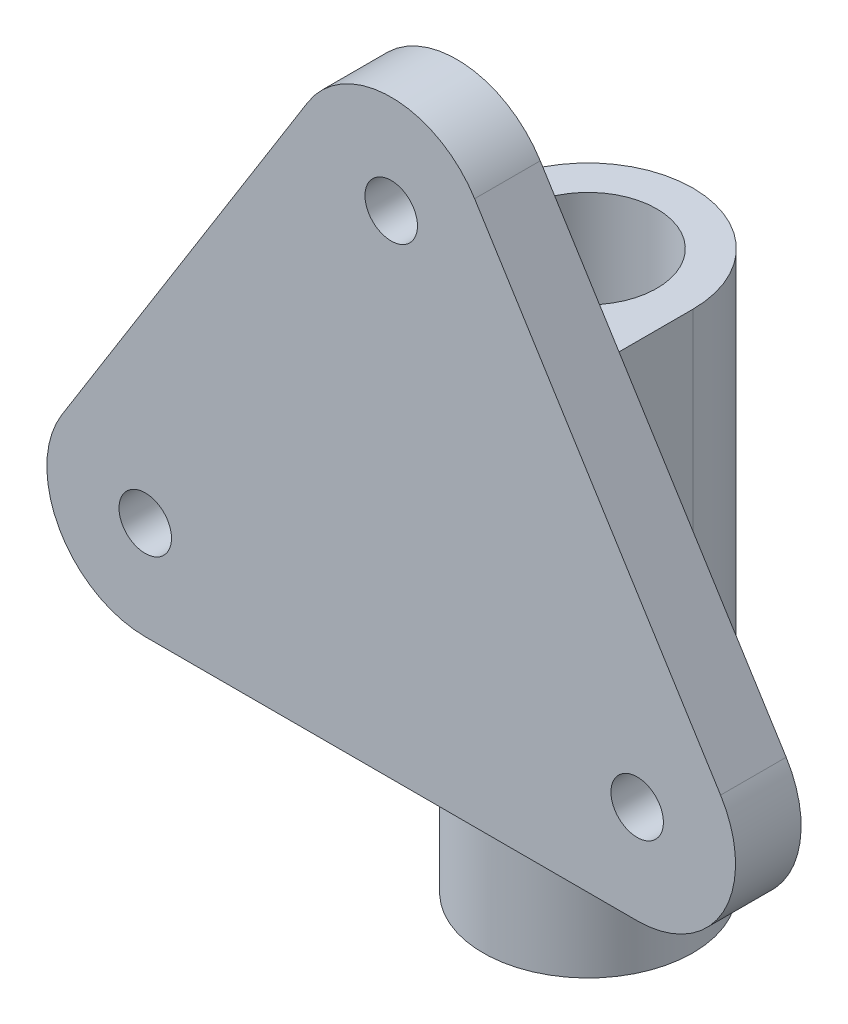
ISO-10303-21;
HEADER;
FILE_DESCRIPTION(('STEP AP214'),'2;1');
FILE_NAME('part.step','',(''),(''),'','','');
FILE_SCHEMA(('AUTOMOTIVE_DESIGN { 1 0 10303 214 1 1 1 1 }'));
ENDSEC;
DATA;
#1=APPLICATION_CONTEXT('core data for automotive mechanical design processes');
#2=APPLICATION_PROTOCOL_DEFINITION('international standard','automotive_design',2000,#1);
#3=PRODUCT_CONTEXT('',#1,'mechanical');
#4=PRODUCT('Part','Part','',(#3));
#5=PRODUCT_RELATED_PRODUCT_CATEGORY('part','',(#4));
#6=PRODUCT_DEFINITION_FORMATION('','',#4);
#7=PRODUCT_DEFINITION_CONTEXT('part definition',#1,'design');
#8=PRODUCT_DEFINITION('design','',#6,#7);
#9=PRODUCT_DEFINITION_SHAPE('','',#8);
#10=(LENGTH_UNIT() NAMED_UNIT(*) SI_UNIT(.MILLI.,.METRE.));
#11=(NAMED_UNIT(*) PLANE_ANGLE_UNIT() SI_UNIT($,.RADIAN.));
#12=(NAMED_UNIT(*) SI_UNIT($,.STERADIAN.) SOLID_ANGLE_UNIT());
#13=UNCERTAINTY_MEASURE_WITH_UNIT(LENGTH_MEASURE(1.E-05),#10,'distance_accuracy_value','');
#14=(GEOMETRIC_REPRESENTATION_CONTEXT(3) GLOBAL_UNCERTAINTY_ASSIGNED_CONTEXT((#13)) GLOBAL_UNIT_ASSIGNED_CONTEXT((#10,
#11,#12)) REPRESENTATION_CONTEXT('',''));
#15=CARTESIAN_POINT('',(0.,0.,0.));
#16=DIRECTION('',(0.,0.,1.));
#17=DIRECTION('',(1.,0.,0.));
#18=AXIS2_PLACEMENT_3D('',#15,#16,#17);
#19=CARTESIAN_POINT('',(-16.,-105.,0.));
#20=DIRECTION('',(1.,0.,0.));
#21=DIRECTION('',(0.,0.,-1.));
#22=AXIS2_PLACEMENT_3D('',#19,#20,#21);
#23=PLANE('',#22);
#24=DIRECTION('',(0.,0.,-1.));
#25=VECTOR('',#24,1.);
#26=CARTESIAN_POINT('',(-16.,-75.,0.));
#27=LINE('',#26,#25);
#28=CARTESIAN_POINT('',(-16.,-75.,0.));
#29=VERTEX_POINT('',#28);
#30=CARTESIAN_POINT('',(-16.,-75.,-20.));
#31=VERTEX_POINT('',#30);
#32=EDGE_CURVE('E191',#29,#31,#27,.T.);
#33=ORIENTED_EDGE('',*,*,#32,.F.);
#34=DIRECTION('',(0.,1.,0.));
#35=VECTOR('',#34,1.);
#36=CARTESIAN_POINT('',(-16.,-60.,0.));
#37=LINE('',#36,#35);
#38=CARTESIAN_POINT('',(-16.,-20.,0.));
#39=VERTEX_POINT('',#38);
#40=EDGE_CURVE('E207',#29,#39,#37,.T.);
#41=ORIENTED_EDGE('',*,*,#40,.T.);
#42=DIRECTION('',(0.,0.,-1.));
#43=VECTOR('',#42,1.);
#44=CARTESIAN_POINT('',(-16.,-20.,0.));
#45=LINE('',#44,#43);
#46=CARTESIAN_POINT('',(-16.,-20.,-20.));
#47=VERTEX_POINT('',#46);
#48=EDGE_CURVE('E232',#39,#47,#45,.T.);
#49=ORIENTED_EDGE('',*,*,#48,.T.);
#50=DIRECTION('',(0.,1.,0.));
#51=VECTOR('',#50,1.);
#52=CARTESIAN_POINT('',(-16.,-105.,-20.));
#53=LINE('',#52,#51);
#54=EDGE_CURVE('E209',#31,#47,#53,.T.);
#55=ORIENTED_EDGE('',*,*,#54,.F.);
#56=EDGE_LOOP('',(#33,#41,#49,#55));
#57=FACE_BOUND('',#56,.T.);
#58=ADVANCED_FACE('F102',(#57),#23,.F.);
#59=CARTESIAN_POINT('',(0.,-105.,0.));
#60=DIRECTION('',(0.,-1.,0.));
#61=DIRECTION('',(0.,0.,-1.));
#62=AXIS2_PLACEMENT_3D('',#59,#60,#61);
#63=PLANE('',#62);
#64=CARTESIAN_POINT('',(0.,-105.,-20.));
#65=DIRECTION('',(0.,-1.,0.));
#66=DIRECTION('',(0.,0.,-1.));
#67=AXIS2_PLACEMENT_3D('',#64,#65,#66);
#68=CIRCLE('',#67,10.5);
#69=CARTESIAN_POINT('',(0.,-105.,-30.5));
#70=VERTEX_POINT('',#69);
#71=EDGE_CURVE('E231',#70,#70,#68,.T.);
#72=ORIENTED_EDGE('',*,*,#71,.F.);
#73=EDGE_LOOP('',(#72));
#74=FACE_BOUND('',#73,.T.);
#75=CARTESIAN_POINT('',(0.,-105.,-20.));
#76=DIRECTION('',(0.,-1.,0.));
#77=DIRECTION('',(0.,0.,-1.));
#78=AXIS2_PLACEMENT_3D('',#75,#76,#77);
#79=CIRCLE('',#78,16.);
#80=CARTESIAN_POINT('',(-16.,-105.,-20.));
#81=VERTEX_POINT('',#80);
#82=CARTESIAN_POINT('',(16.,-105.,-20.));
#83=VERTEX_POINT('',#82);
#84=EDGE_CURVE('E213',#81,#83,#79,.T.);
#85=ORIENTED_EDGE('',*,*,#84,.T.);
#86=CARTESIAN_POINT('',(16.,-105.,-20.));
#87=CARTESIAN_POINT('',(16.,-105.,-16.8176750296418));
#88=CARTESIAN_POINT('',(14.7820725201806,-105.,-13.8770650821586));
#89=CARTESIAN_POINT('',(13.5644424143641,-105.,-10.9371731256605));
#90=CARTESIAN_POINT('',(11.3137084989848,-105.,-8.68629150101524));
#91=CARTESIAN_POINT('',(9.06371702136959,-105.,-6.43615236285823));
#92=CARTESIAN_POINT('',(6.12293491784144,-105.,-5.21792747981942));
#93=CARTESIAN_POINT('',(3.18312287464358,-105.,-4.00010444621753));
#94=CARTESIAN_POINT('',(0.,-105.,-4.));
#95=CARTESIAN_POINT('',(-3.18207287466311,-105.,-3.9998955882356));
#96=CARTESIAN_POINT('',(-6.12293491784143,-105.,-5.21792747981941));
#97=CARTESIAN_POINT('',(-9.0628268743386,-105.,-6.435557585635));
#98=CARTESIAN_POINT('',(-11.3137084989848,-105.,-8.68629150101524));
#99=CARTESIAN_POINT('',(-13.5638476371406,-105.,-10.9362829786292));
#100=CARTESIAN_POINT('',(-14.7820725201806,-105.,-13.8770650821586));
#101=CARTESIAN_POINT('',(-16.,-105.,-16.8171292574295));
#102=CARTESIAN_POINT('',(-16.,-105.,-20.));
#103=B_SPLINE_CURVE_WITH_KNOTS('',2,(#86,#87,#88,#89,#90,#91,#92,#93,#94,#95,#96,#97,#98,#99,
#100,#101,#102),.UNSPECIFIED.,.F.,.F.,(3,2,2,2,2,2,2,2,3),(0.,0.125,0.25,0.375,0.5,0.625,0.75,
0.875,1.),.UNSPECIFIED.);
#104=EDGE_CURVE('E228',#83,#81,#103,.T.);
#105=ORIENTED_EDGE('',*,*,#104,.T.);
#106=EDGE_LOOP('',(#85,#105));
#107=FACE_BOUND('',#106,.T.);
#108=ADVANCED_FACE('F233',(#74,#107),#63,.T.);
#109=CARTESIAN_POINT('',(37.5,-60.,10.));
#110=DIRECTION('',(0.,0.,1.));
#111=DIRECTION('',(1.,0.,0.));
#112=AXIS2_PLACEMENT_3D('',#109,#110,#111);
#113=PLANE('',#112);
#114=DIRECTION('',(1.,0.,0.));
#115=VECTOR('',#114,1.);
#116=CARTESIAN_POINT('',(-37.5,-75.,10.));
#117=LINE('',#116,#115);
#118=CARTESIAN_POINT('',(-37.5,-75.,10.));
#119=VERTEX_POINT('',#118);
#120=CARTESIAN_POINT('',(37.5,-75.,10.));
#121=VERTEX_POINT('',#120);
#122=EDGE_CURVE('E258',#119,#121,#117,.T.);
#123=ORIENTED_EDGE('',*,*,#122,.T.);
#124=CARTESIAN_POINT('',(37.5,-60.,10.));
#125=DIRECTION('',(0.,0.,1.));
#126=DIRECTION('',(1.,0.,0.));
#127=AXIS2_PLACEMENT_3D('',#124,#125,#126);
#128=CIRCLE('',#127,15.);
#129=CARTESIAN_POINT('',(50.2199745600763,-52.0500158999523,10.));
#130=VERTEX_POINT('',#129);
#131=EDGE_CURVE('E279',#121,#130,#128,.T.);
#132=ORIENTED_EDGE('',*,*,#131,.T.);
#133=DIRECTION('',(0.52999894000318,-0.847998304005088,0.));
#134=VECTOR('',#133,1.);
#135=CARTESIAN_POINT('',(12.7199745600763,7.9499841000477,10.));
#136=LINE('',#135,#134);
#137=CARTESIAN_POINT('',(12.7199745600763,7.9499841000477,10.));
#138=VERTEX_POINT('',#137);
#139=EDGE_CURVE('E274',#138,#130,#136,.T.);
#140=ORIENTED_EDGE('',*,*,#139,.F.);
#141=CARTESIAN_POINT('',(0.,0.,10.));
#142=DIRECTION('',(0.,0.,1.));
#143=DIRECTION('',(1.,0.,0.));
#144=AXIS2_PLACEMENT_3D('',#141,#142,#143);
#145=CIRCLE('',#144,15.);
#146=CARTESIAN_POINT('',(-12.7199745600763,7.9499841000477,10.));
#147=VERTEX_POINT('',#146);
#148=EDGE_CURVE('E272',#138,#147,#145,.T.);
#149=ORIENTED_EDGE('',*,*,#148,.T.);
#150=DIRECTION('',(-0.52999894000318,-0.847998304005088,0.));
#151=VECTOR('',#150,1.);
#152=CARTESIAN_POINT('',(-12.7199745600763,7.9499841000477,10.));
#153=LINE('',#152,#151);
#154=CARTESIAN_POINT('',(-50.2199745600763,-52.0500158999523,10.));
#155=VERTEX_POINT('',#154);
#156=EDGE_CURVE('E271',#147,#155,#153,.T.);
#157=ORIENTED_EDGE('',*,*,#156,.T.);
#158=CARTESIAN_POINT('',(-37.5,-60.,10.));
#159=DIRECTION('',(0.,0.,1.));
#160=DIRECTION('',(1.,0.,0.));
#161=AXIS2_PLACEMENT_3D('',#158,#159,#160);
#162=CIRCLE('',#161,15.);
#163=EDGE_CURVE('E251',#155,#119,#162,.T.);
#164=ORIENTED_EDGE('',*,*,#163,.T.);
#165=EDGE_LOOP('',(#123,#132,#140,#149,#157,#164));
#166=FACE_BOUND('',#165,.T.);
#167=CARTESIAN_POINT('',(-37.5,-60.,10.));
#168=DIRECTION('',(0.,0.,1.));
#169=DIRECTION('',(1.,0.,0.));
#170=AXIS2_PLACEMENT_3D('',#167,#168,#169);
#171=CIRCLE('',#170,4.00000000000002);
#172=CARTESIAN_POINT('',(-33.5,-60.,10.));
#173=VERTEX_POINT('',#172);
#174=EDGE_CURVE('E284',#173,#173,#171,.T.);
#175=ORIENTED_EDGE('',*,*,#174,.F.);
#176=EDGE_LOOP('',(#175));
#177=FACE_BOUND('',#176,.T.);
#178=CARTESIAN_POINT('',(0.,0.,10.));
#179=DIRECTION('',(0.,0.,1.));
#180=DIRECTION('',(1.,0.,0.));
#181=AXIS2_PLACEMENT_3D('',#178,#179,#180);
#182=CIRCLE('',#181,4.);
#183=CARTESIAN_POINT('',(4.,0.,10.));
#184=VERTEX_POINT('',#183);
#185=EDGE_CURVE('E283',#184,#184,#182,.T.);
#186=ORIENTED_EDGE('',*,*,#185,.F.);
#187=EDGE_LOOP('',(#186));
#188=FACE_BOUND('',#187,.T.);
#189=CARTESIAN_POINT('',(37.5,-60.,10.));
#190=DIRECTION('',(0.,0.,1.));
#191=DIRECTION('',(1.,0.,0.));
#192=AXIS2_PLACEMENT_3D('',#189,#190,#191);
#193=CIRCLE('',#192,4.00000000000002);
#194=CARTESIAN_POINT('',(41.5,-60.,10.));
#195=VERTEX_POINT('',#194);
#196=EDGE_CURVE('E292',#195,#195,#193,.T.);
#197=ORIENTED_EDGE('',*,*,#196,.F.);
#198=EDGE_LOOP('',(#197));
#199=FACE_BOUND('',#198,.T.);
#200=ADVANCED_FACE('F330',(#166,#177,#188,#199),#113,.T.);
#201=CARTESIAN_POINT('',(37.5,-60.,0.));
#202=DIRECTION('',(0.,0.,1.));
#203=DIRECTION('',(1.,0.,0.));
#204=AXIS2_PLACEMENT_3D('',#201,#202,#203);
#205=PLANE('',#204);
#206=DIRECTION('',(1.,0.,0.));
#207=VECTOR('',#206,1.);
#208=CARTESIAN_POINT('',(-37.5,-75.,0.));
#209=LINE('',#208,#207);
#210=CARTESIAN_POINT('',(16.,-75.,0.));
#211=VERTEX_POINT('',#210);
#212=CARTESIAN_POINT('',(37.5,-75.,0.));
#213=VERTEX_POINT('',#212);
#214=EDGE_CURVE('E267',#211,#213,#209,.T.);
#215=ORIENTED_EDGE('',*,*,#214,.F.);
#216=DIRECTION('',(0.,1.,0.));
#217=VECTOR('',#216,1.);
#218=CARTESIAN_POINT('',(16.,-60.,0.));
#219=LINE('',#218,#217);
#220=CARTESIAN_POINT('',(16.,-20.,0.));
#221=VERTEX_POINT('',#220);
#222=EDGE_CURVE('E121',#211,#221,#219,.T.);
#223=ORIENTED_EDGE('',*,*,#222,.T.);
#224=DIRECTION('',(1.,0.,0.));
#225=VECTOR('',#224,1.);
#226=CARTESIAN_POINT('',(37.5,-20.,0.));
#227=LINE('',#226,#225);
#228=EDGE_CURVE('E12',#39,#221,#227,.T.);
#229=ORIENTED_EDGE('',*,*,#228,.F.);
#230=ORIENTED_EDGE('',*,*,#40,.F.);
#231=CARTESIAN_POINT('',(-37.5,-75.,0.));
#232=VERTEX_POINT('',#231);
#233=EDGE_CURVE('E270',#232,#29,#209,.T.);
#234=ORIENTED_EDGE('',*,*,#233,.F.);
#235=CARTESIAN_POINT('',(-37.5,-60.,0.));
#236=DIRECTION('',(0.,0.,1.));
#237=DIRECTION('',(1.,0.,0.));
#238=AXIS2_PLACEMENT_3D('',#235,#236,#237);
#239=CIRCLE('',#238,15.);
#240=CARTESIAN_POINT('',(-50.2199745600763,-52.0500158999523,0.));
#241=VERTEX_POINT('',#240);
#242=EDGE_CURVE('E255',#241,#232,#239,.T.);
#243=ORIENTED_EDGE('',*,*,#242,.F.);
#244=DIRECTION('',(-0.52999894000318,-0.847998304005088,0.));
#245=VECTOR('',#244,1.);
#246=CARTESIAN_POINT('',(-12.7199745600763,7.9499841000477,0.));
#247=LINE('',#246,#245);
#248=CARTESIAN_POINT('',(-12.7199745600763,7.9499841000477,0.));
#249=VERTEX_POINT('',#248);
#250=EDGE_CURVE('E260',#249,#241,#247,.T.);
#251=ORIENTED_EDGE('',*,*,#250,.F.);
#252=CARTESIAN_POINT('',(0.,0.,0.));
#253=DIRECTION('',(0.,0.,1.));
#254=DIRECTION('',(1.,0.,0.));
#255=AXIS2_PLACEMENT_3D('',#252,#253,#254);
#256=CIRCLE('',#255,15.);
#257=CARTESIAN_POINT('',(12.7199745600763,7.9499841000477,0.));
#258=VERTEX_POINT('',#257);
#259=EDGE_CURVE('E259',#258,#249,#256,.T.);
#260=ORIENTED_EDGE('',*,*,#259,.F.);
#261=DIRECTION('',(0.52999894000318,-0.847998304005088,0.));
#262=VECTOR('',#261,1.);
#263=CARTESIAN_POINT('',(12.7199745600763,7.9499841000477,0.));
#264=LINE('',#263,#262);
#265=CARTESIAN_POINT('',(50.2199745600763,-52.0500158999523,0.));
#266=VERTEX_POINT('',#265);
#267=EDGE_CURVE('E261',#258,#266,#264,.T.);
#268=ORIENTED_EDGE('',*,*,#267,.T.);
#269=CARTESIAN_POINT('',(37.5,-60.,0.));
#270=DIRECTION('',(0.,0.,1.));
#271=DIRECTION('',(1.,0.,0.));
#272=AXIS2_PLACEMENT_3D('',#269,#270,#271);
#273=CIRCLE('',#272,15.);
#274=EDGE_CURVE('E262',#213,#266,#273,.T.);
#275=ORIENTED_EDGE('',*,*,#274,.F.);
#276=EDGE_LOOP('',(#215,#223,#229,#230,#234,#243,#251,#260,#268,#275));
#277=FACE_BOUND('',#276,.T.);
#278=CARTESIAN_POINT('',(0.,0.,0.));
#279=DIRECTION('',(0.,0.,1.));
#280=DIRECTION('',(1.,0.,0.));
#281=AXIS2_PLACEMENT_3D('',#278,#279,#280);
#282=CIRCLE('',#281,4.);
#283=CARTESIAN_POINT('',(4.,0.,0.));
#284=VERTEX_POINT('',#283);
#285=EDGE_CURVE('E281',#284,#284,#282,.T.);
#286=ORIENTED_EDGE('',*,*,#285,.T.);
#287=EDGE_LOOP('',(#286));
#288=FACE_BOUND('',#287,.T.);
#289=CARTESIAN_POINT('',(-37.5,-60.,0.));
#290=DIRECTION('',(0.,0.,1.));
#291=DIRECTION('',(1.,0.,0.));
#292=AXIS2_PLACEMENT_3D('',#289,#290,#291);
#293=CIRCLE('',#292,4.00000000000002);
#294=CARTESIAN_POINT('',(-33.5,-60.,0.));
#295=VERTEX_POINT('',#294);
#296=EDGE_CURVE('E286',#295,#295,#293,.T.);
#297=ORIENTED_EDGE('',*,*,#296,.T.);
#298=EDGE_LOOP('',(#297));
#299=FACE_BOUND('',#298,.T.);
#300=CARTESIAN_POINT('',(37.5,-60.,0.));
#301=DIRECTION('',(0.,0.,1.));
#302=DIRECTION('',(1.,0.,0.));
#303=AXIS2_PLACEMENT_3D('',#300,#301,#302);
#304=CIRCLE('',#303,4.00000000000002);
#305=CARTESIAN_POINT('',(41.5,-60.,0.));
#306=VERTEX_POINT('',#305);
#307=EDGE_CURVE('E294',#306,#306,#304,.T.);
#308=ORIENTED_EDGE('',*,*,#307,.T.);
#309=EDGE_LOOP('',(#308));
#310=FACE_BOUND('',#309,.T.);
#311=ADVANCED_FACE('F358',(#277,#288,#299,#310),#205,.F.);
#312=CARTESIAN_POINT('',(-37.5,-75.,10.));
#313=DIRECTION('',(0.,1.,0.));
#314=DIRECTION('',(0.,0.,1.));
#315=AXIS2_PLACEMENT_3D('',#312,#313,#314);
#316=PLANE('',#315);
#317=DIRECTION('',(0.,0.,-1.));
#318=VECTOR('',#317,1.);
#319=CARTESIAN_POINT('',(37.5,-75.,10.));
#320=LINE('',#319,#318);
#321=EDGE_CURVE('E113',#121,#213,#320,.T.);
#322=ORIENTED_EDGE('',*,*,#321,.F.);
#323=ORIENTED_EDGE('',*,*,#122,.F.);
#324=DIRECTION('',(0.,0.,-1.));
#325=VECTOR('',#324,1.);
#326=CARTESIAN_POINT('',(-37.5,-75.,10.));
#327=LINE('',#326,#325);
#328=EDGE_CURVE('E247',#119,#232,#327,.T.);
#329=ORIENTED_EDGE('',*,*,#328,.T.);
#330=ORIENTED_EDGE('',*,*,#233,.T.);
#331=ORIENTED_EDGE('',*,*,#32,.T.);
#332=CARTESIAN_POINT('',(0.,-75.,-20.));
#333=DIRECTION('',(0.,-1.,0.));
#334=DIRECTION('',(0.,0.,-1.));
#335=AXIS2_PLACEMENT_3D('',#332,#333,#334);
#336=CIRCLE('',#335,16.);
#337=CARTESIAN_POINT('',(16.,-75.,-20.));
#338=VERTEX_POINT('',#337);
#339=EDGE_CURVE('E187',#338,#31,#336,.T.);
#340=ORIENTED_EDGE('',*,*,#339,.F.);
#341=DIRECTION('',(0.,0.,1.));
#342=VECTOR('',#341,1.);
#343=CARTESIAN_POINT('',(16.,-75.,0.));
#344=LINE('',#343,#342);
#345=EDGE_CURVE('E193',#338,#211,#344,.T.);
#346=ORIENTED_EDGE('',*,*,#345,.T.);
#347=ORIENTED_EDGE('',*,*,#214,.T.);
#348=EDGE_LOOP('',(#322,#323,#329,#330,#331,#340,#346,#347));
#349=FACE_BOUND('',#348,.T.);
#350=ADVANCED_FACE('F106',(#349),#316,.F.);
#351=CARTESIAN_POINT('',(37.5,-60.,10.));
#352=DIRECTION('',(0.,0.,-1.));
#353=DIRECTION('',(-1.,0.,0.));
#354=AXIS2_PLACEMENT_3D('',#351,#352,#353);
#355=CYLINDRICAL_SURFACE('',#354,15.);
#356=ORIENTED_EDGE('',*,*,#274,.T.);
#357=DIRECTION('',(0.,0.,-1.));
#358=VECTOR('',#357,1.);
#359=CARTESIAN_POINT('',(50.2199745600763,-52.0500158999523,10.));
#360=LINE('',#359,#358);
#361=EDGE_CURVE('E238',#130,#266,#360,.T.);
#362=ORIENTED_EDGE('',*,*,#361,.F.);
#363=ORIENTED_EDGE('',*,*,#131,.F.);
#364=ORIENTED_EDGE('',*,*,#321,.T.);
#365=EDGE_LOOP('',(#356,#362,#363,#364));
#366=FACE_BOUND('',#365,.T.);
#367=ADVANCED_FACE('F373',(#366),#355,.T.);
#368=CARTESIAN_POINT('',(12.7199745600763,7.9499841000477,10.));
#369=DIRECTION('',(0.847998304005088,0.52999894000318,0.));
#370=DIRECTION('',(-0.52999894000318,0.847998304005088,0.));
#371=AXIS2_PLACEMENT_3D('',#368,#369,#370);
#372=PLANE('',#371);
#373=ORIENTED_EDGE('',*,*,#267,.F.);
#374=DIRECTION('',(0.,0.,-1.));
#375=VECTOR('',#374,1.);
#376=CARTESIAN_POINT('',(12.7199745600763,7.9499841000477,10.));
#377=LINE('',#376,#375);
#378=EDGE_CURVE('E245',#138,#258,#377,.T.);
#379=ORIENTED_EDGE('',*,*,#378,.F.);
#380=ORIENTED_EDGE('',*,*,#139,.T.);
#381=ORIENTED_EDGE('',*,*,#361,.T.);
#382=EDGE_LOOP('',(#373,#379,#380,#381));
#383=FACE_BOUND('',#382,.T.);
#384=ADVANCED_FACE('F367',(#383),#372,.T.);
#385=CARTESIAN_POINT('',(0.,0.,10.));
#386=DIRECTION('',(0.,0.,-1.));
#387=DIRECTION('',(-1.,0.,0.));
#388=AXIS2_PLACEMENT_3D('',#385,#386,#387);
#389=CYLINDRICAL_SURFACE('',#388,15.);
#390=ORIENTED_EDGE('',*,*,#259,.T.);
#391=DIRECTION('',(0.,0.,-1.));
#392=VECTOR('',#391,1.);
#393=CARTESIAN_POINT('',(-12.7199745600763,7.9499841000477,10.));
#394=LINE('',#393,#392);
#395=EDGE_CURVE('E243',#147,#249,#394,.T.);
#396=ORIENTED_EDGE('',*,*,#395,.F.);
#397=ORIENTED_EDGE('',*,*,#148,.F.);
#398=ORIENTED_EDGE('',*,*,#378,.T.);
#399=EDGE_LOOP('',(#390,#396,#397,#398));
#400=FACE_BOUND('',#399,.T.);
#401=ADVANCED_FACE('F368',(#400),#389,.T.);
#402=CARTESIAN_POINT('',(-12.7199745600763,7.9499841000477,10.));
#403=DIRECTION('',(0.847998304005088,-0.52999894000318,0.));
#404=DIRECTION('',(0.52999894000318,0.847998304005088,0.));
#405=AXIS2_PLACEMENT_3D('',#402,#403,#404);
#406=PLANE('',#405);
#407=ORIENTED_EDGE('',*,*,#250,.T.);
#408=DIRECTION('',(0.,0.,-1.));
#409=VECTOR('',#408,1.);
#410=CARTESIAN_POINT('',(-50.2199745600763,-52.0500158999523,10.));
#411=LINE('',#410,#409);
#412=EDGE_CURVE('E250',#155,#241,#411,.T.);
#413=ORIENTED_EDGE('',*,*,#412,.F.);
#414=ORIENTED_EDGE('',*,*,#156,.F.);
#415=ORIENTED_EDGE('',*,*,#395,.T.);
#416=EDGE_LOOP('',(#407,#413,#414,#415));
#417=FACE_BOUND('',#416,.T.);
#418=ADVANCED_FACE('F362',(#417),#406,.F.);
#419=CARTESIAN_POINT('',(-37.5,-60.,10.));
#420=DIRECTION('',(0.,0.,-1.));
#421=DIRECTION('',(-1.,0.,0.));
#422=AXIS2_PLACEMENT_3D('',#419,#420,#421);
#423=CYLINDRICAL_SURFACE('',#422,15.);
#424=ORIENTED_EDGE('',*,*,#242,.T.);
#425=ORIENTED_EDGE('',*,*,#328,.F.);
#426=ORIENTED_EDGE('',*,*,#163,.F.);
#427=ORIENTED_EDGE('',*,*,#412,.T.);
#428=EDGE_LOOP('',(#424,#425,#426,#427));
#429=FACE_BOUND('',#428,.T.);
#430=ADVANCED_FACE('F355',(#429),#423,.T.);
#431=CARTESIAN_POINT('',(0.,0.,10.));
#432=DIRECTION('',(0.,0.,-1.));
#433=DIRECTION('',(-1.,0.,0.));
#434=AXIS2_PLACEMENT_3D('',#431,#432,#433);
#435=CYLINDRICAL_SURFACE('',#434,4.);
#436=ORIENTED_EDGE('',*,*,#185,.T.);
#437=EDGE_LOOP('',(#436));
#438=FACE_BOUND('',#437,.T.);
#439=ORIENTED_EDGE('',*,*,#285,.F.);
#440=EDGE_LOOP('',(#439));
#441=FACE_BOUND('',#440,.T.);
#442=ADVANCED_FACE('F342',(#438,#441),#435,.F.);
#443=CARTESIAN_POINT('',(-37.5,-60.,10.));
#444=DIRECTION('',(0.,0.,-1.));
#445=DIRECTION('',(-1.,0.,0.));
#446=AXIS2_PLACEMENT_3D('',#443,#444,#445);
#447=CYLINDRICAL_SURFACE('',#446,4.00000000000002);
#448=ORIENTED_EDGE('',*,*,#174,.T.);
#449=EDGE_LOOP('',(#448));
#450=FACE_BOUND('',#449,.T.);
#451=ORIENTED_EDGE('',*,*,#296,.F.);
#452=EDGE_LOOP('',(#451));
#453=FACE_BOUND('',#452,.T.);
#454=ADVANCED_FACE('F339',(#450,#453),#447,.F.);
#455=CARTESIAN_POINT('',(37.5,-60.,10.));
#456=DIRECTION('',(0.,0.,-1.));
#457=DIRECTION('',(-1.,0.,0.));
#458=AXIS2_PLACEMENT_3D('',#455,#456,#457);
#459=CYLINDRICAL_SURFACE('',#458,4.00000000000002);
#460=ORIENTED_EDGE('',*,*,#196,.T.);
#461=EDGE_LOOP('',(#460));
#462=FACE_BOUND('',#461,.T.);
#463=ORIENTED_EDGE('',*,*,#307,.F.);
#464=EDGE_LOOP('',(#463));
#465=FACE_BOUND('',#464,.T.);
#466=ADVANCED_FACE('F336',(#462,#465),#459,.F.);
#467=CARTESIAN_POINT('',(0.,-20.,0.));
#468=DIRECTION('',(0.,-1.,0.));
#469=DIRECTION('',(0.,0.,-1.));
#470=AXIS2_PLACEMENT_3D('',#467,#468,#469);
#471=PLANE('',#470);
#472=CARTESIAN_POINT('',(0.,-20.,-20.));
#473=DIRECTION('',(0.,-1.,0.));
#474=DIRECTION('',(0.,0.,-1.));
#475=AXIS2_PLACEMENT_3D('',#472,#473,#474);
#476=CIRCLE('',#475,10.5);
#477=CARTESIAN_POINT('',(0.,-20.,-30.5));
#478=VERTEX_POINT('',#477);
#479=EDGE_CURVE('E235',#478,#478,#476,.T.);
#480=ORIENTED_EDGE('',*,*,#479,.T.);
#481=EDGE_LOOP('',(#480));
#482=FACE_BOUND('',#481,.T.);
#483=ORIENTED_EDGE('',*,*,#48,.F.);
#484=ORIENTED_EDGE('',*,*,#228,.T.);
#485=DIRECTION('',(0.,0.,-1.));
#486=VECTOR('',#485,1.);
#487=CARTESIAN_POINT('',(16.,-20.,0.));
#488=LINE('',#487,#486);
#489=CARTESIAN_POINT('',(16.,-20.,-20.));
#490=VERTEX_POINT('',#489);
#491=EDGE_CURVE('E305',#221,#490,#488,.T.);
#492=ORIENTED_EDGE('',*,*,#491,.T.);
#493=CARTESIAN_POINT('',(0.,-20.,-20.));
#494=DIRECTION('',(0.,-1.,0.));
#495=DIRECTION('',(0.,0.,-1.));
#496=AXIS2_PLACEMENT_3D('',#493,#494,#495);
#497=CIRCLE('',#496,16.);
#498=EDGE_CURVE('E208',#47,#490,#497,.T.);
#499=ORIENTED_EDGE('',*,*,#498,.F.);
#500=EDGE_LOOP('',(#483,#484,#492,#499));
#501=FACE_BOUND('',#500,.T.);
#502=ADVANCED_FACE('F310',(#482,#501),#471,.F.);
#503=CARTESIAN_POINT('',(16.,-105.,0.));
#504=DIRECTION('',(1.,0.,0.));
#505=DIRECTION('',(0.,0.,-1.));
#506=AXIS2_PLACEMENT_3D('',#503,#504,#505);
#507=PLANE('',#506);
#508=ORIENTED_EDGE('',*,*,#345,.F.);
#509=DIRECTION('',(0.,1.,0.));
#510=VECTOR('',#509,1.);
#511=CARTESIAN_POINT('',(16.,-105.,-20.));
#512=LINE('',#511,#510);
#513=EDGE_CURVE('E203',#338,#490,#512,.T.);
#514=ORIENTED_EDGE('',*,*,#513,.T.);
#515=ORIENTED_EDGE('',*,*,#491,.F.);
#516=ORIENTED_EDGE('',*,*,#222,.F.);
#517=EDGE_LOOP('',(#508,#514,#515,#516));
#518=FACE_BOUND('',#517,.T.);
#519=ADVANCED_FACE('F200',(#518),#507,.T.);
#520=CARTESIAN_POINT('',(0.,-105.,-20.));
#521=DIRECTION('',(0.,1.,0.));
#522=DIRECTION('',(0.,0.,1.));
#523=AXIS2_PLACEMENT_3D('',#520,#521,#522);
#524=CYLINDRICAL_SURFACE('',#523,16.);
#525=ORIENTED_EDGE('',*,*,#513,.F.);
#526=ORIENTED_EDGE('',*,*,#339,.T.);
#527=ORIENTED_EDGE('',*,*,#54,.T.);
#528=ORIENTED_EDGE('',*,*,#498,.T.);
#529=EDGE_LOOP('',(#525,#526,#527,#528));
#530=FACE_BOUND('',#529,.T.);
#531=ORIENTED_EDGE('',*,*,#104,.F.);
#532=ORIENTED_EDGE('',*,*,#84,.F.);
#533=EDGE_LOOP('',(#531,#532));
#534=FACE_BOUND('',#533,.T.);
#535=ADVANCED_FACE('F202',(#530,#534),#524,.T.);
#536=CARTESIAN_POINT('',(0.,-105.,-20.));
#537=DIRECTION('',(0.,1.,0.));
#538=DIRECTION('',(0.,0.,1.));
#539=AXIS2_PLACEMENT_3D('',#536,#537,#538);
#540=CYLINDRICAL_SURFACE('',#539,10.5);
#541=ORIENTED_EDGE('',*,*,#71,.T.);
#542=EDGE_LOOP('',(#541));
#543=FACE_BOUND('',#542,.T.);
#544=ORIENTED_EDGE('',*,*,#479,.F.);
#545=EDGE_LOOP('',(#544));
#546=FACE_BOUND('',#545,.T.);
#547=ADVANCED_FACE('F315',(#543,#546),#540,.F.);
#548=CLOSED_SHELL('',(#58,#108,#200,#311,#350,#367,#384,#401,#418,#430,#442,#454,#466,#502,#519,
#535,#547));
#549=MANIFOLD_SOLID_BREP('B2',#548);
#550=ADVANCED_BREP_SHAPE_REPRESENTATION('',(#18,#549),#14);
#551=SHAPE_DEFINITION_REPRESENTATION(#9,#550);
ENDSEC;
END-ISO-10303-21;
